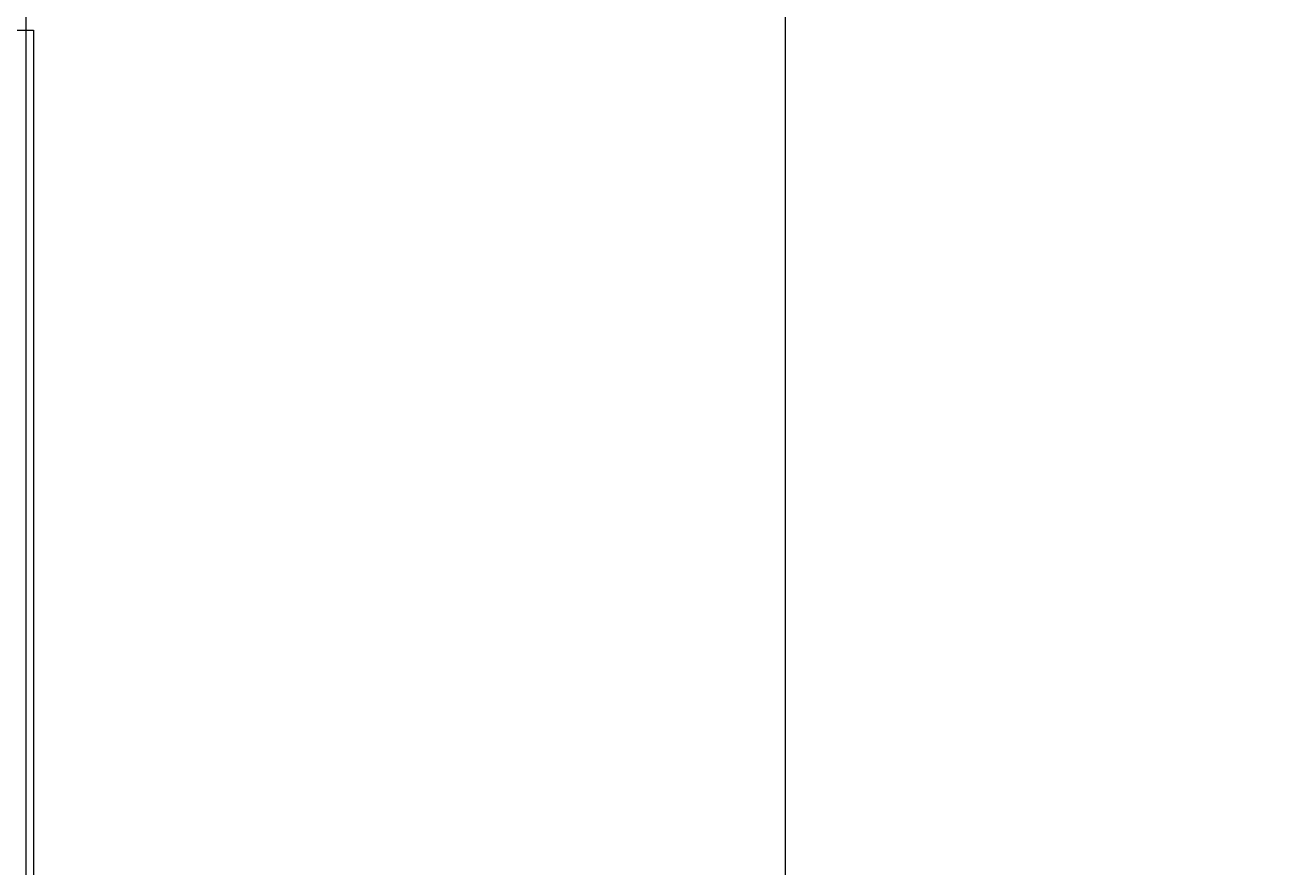
# Model space of a CAD drawing. Units: millimetres. Extents: x 27017497 to 27018854, y 7058029 to 7059154.
# Tile 13 of 91: x 27017623 to 27017651, y 7058219 to 7058238. Entities that reach past the tile are written whole.
import ezdxf

# ---------------------------------------------------------------- set-up
doc = ezdxf.new("R2010")
doc.units = ezdxf.units.MM
for name, color, linetype, lineweight in [('A-ANNO-DIMS', 2, 'Continuous', 18), ('A-FLOR-CASE', 8, 'Continuous', 20), ('A-GLAZ', 4, 'Continuous', 18)]:
    doc.layers.add(name, color=color, linetype=linetype, lineweight=lineweight)
doc.styles.get("Standard").update_dxf_attribs({"font": 'arial.ttf'})
doc.dimstyles.get("Standard").update_dxf_attribs({"dimtxt": 0.18, "dimasz": 0.18, "dimexe": 0.18, "dimexo": 0.0625, "dimgap": 0.09, "dimtad": 0, "dimtih": 1, "dimtoh": 1, "dimdec": 4, "dimzin": 0, "dimdsep": 46, "dimtxsty": 'Standard', "dimcen": 0.09, "dimadec": 0, "dimazin": 0, "dimtfac": 1, "dimtdec": 4, "dimtofl": 0, "dimtmove": 0, "dimatfit": 3, "dimfxl": 1, "dimtolj": 1, "dimtzin": 0, "dimarcsym": 0})

# ---------------------------------------------------------------- blocks, each defined once
blk = doc.blocks.new('WINDOW-SINGLE-LIGHT')
blk.add_lwpolyline([(36, 4.5), (36, 0), (0, 0), (0, 9), (36, 9), (36, 4.5), (0, 4.5)])
blk = doc.blocks.new('*D47')
at = {"layer": 'A-ANNO-DIMS', "color": 0, "lineweight": -2, "transparency": 16777216}
for p, q in [((27017561.166, 7058294.35), (27017561.166, 7058028.6)), ((27018790.606, 7058294.35), (27018790.606, 7058028.6)), ((27017561.346, 7058028.78), (27018175.431, 7058028.78)), ((27018790.426, 7058028.78), (27018176.341, 7058028.78))]:
    blk.add_line(p, q, dxfattribs=at)
at = {"layer": 'A-ANNO-DIMS', "color": 0, "transparency": 16777216}
for points in [[(27017561.346, 7058028.81), (27017561.346, 7058028.75), (27017561.166, 7058028.78)], [(27018790.426, 7058028.81), (27018790.426, 7058028.75), (27018790.606, 7058028.78)]]:
    blk.add_solid(points, dxfattribs=at)
at = {"layer": 'Defpoints', "color": 0, "transparency": 16777216}
for p in [(27017561.166, 7058294.412), (27018790.606, 7058294.412), (27018790.606, 7058028.78)]:
    blk.add_point(p, dxfattribs=at)
at = {"layer": 'A-ANNO-DIMS', "color": 0, "transparency": 16777216, "insert": (27018175.886, 7058028.78), "char_height": 0.18, "attachment_point": 5}
blk.add_mtext('\\A1;1229.4', dxfattribs=at)
blk = doc.blocks.new('*D48')
at = {"layer": 'A-ANNO-DIMS', "color": 0, "lineweight": -2, "transparency": 16777216}
for p, q in [((27018463.498, 7058622.912), (27017497.536, 7058622.912)), ((27017497.716, 7058622.732), (27017497.716, 7058357.753)), ((27017497.716, 7058092.41), (27017497.716, 7058357.389)), ((27018555.129, 7058092.23), (27017497.536, 7058092.23))]:
    blk.add_line(p, q, dxfattribs=at)
at = {"layer": 'A-ANNO-DIMS', "color": 0, "transparency": 16777216}
for points in [[(27017497.686, 7058622.732), (27017497.746, 7058622.732), (27017497.716, 7058622.912)], [(27017497.686, 7058092.41), (27017497.746, 7058092.41), (27017497.716, 7058092.23)]]:
    blk.add_solid(points, dxfattribs=at)
at = {"layer": 'Defpoints', "color": 0, "transparency": 16777216}
for p in [(27018463.561, 7058622.912), (27017497.716, 7058092.23), (27018555.192, 7058092.23)]:
    blk.add_point(p, dxfattribs=at)
at = {"layer": 'A-ANNO-DIMS', "color": 0, "transparency": 16777216, "insert": (27017497.716, 7058357.571), "char_height": 0.18, "attachment_point": 5}
blk.add_mtext('\\A1;530.7', dxfattribs=at)

msp = doc.modelspace()

# ---------------------------------------------------------------- linework, layer by layer
at = {"layer": 'A-FLOR-CASE'}
for p, q in [((27017639.716, 7058294.412), (27017639.716, 7058207.055)), ((27017622.691, 7058258.237), (27017622.691, 7058207.055))]:
    msp.add_line(p, q, dxfattribs=at)

# ---------------------------------------------------------------- block references
at = {"layer": 'A-GLAZ', "rotation": 270}
msp.add_blockref('WINDOW-SINGLE-LIGHT', (27017613.865, 7058237.7), dxfattribs=at)

# ---------------------------------------------------------------- dimensions: what is measured, and where the dimension line sits
at = {"layer": 'A-ANNO-DIMS'}
dim = msp.add_linear_dim(base=(27017497.716, 7058092.23), p1=(27018463.561, 7058622.912), p2=(27018555.192, 7058092.23), angle=90, dimstyle='Standard', override={"dimdec": 1, "dimlfac": 1, "dimrnd": 0, "dimzin": 0, "dimdsep": 46, "dimlunit": 2}, dxfattribs=at)
dim.commit()
dim.dimension.update_dxf_attribs({"geometry": '*D48', "text_midpoint": (27017497.716, 7058357.571)})
dim = msp.add_linear_dim(base=(27018790.606, 7058028.78), p1=(27017561.166, 7058294.412), p2=(27018790.606, 7058294.412), dimstyle='Standard', override={"dimdec": 1, "dimlfac": 1, "dimrnd": 0, "dimzin": 0, "dimdsep": 46, "dimlunit": 2}, dxfattribs=at)
dim.commit()
dim.dimension.update_dxf_attribs({"geometry": '*D47', "text_midpoint": (27018175.886, 7058028.78)})

doc.saveas('drawing.dxf')
